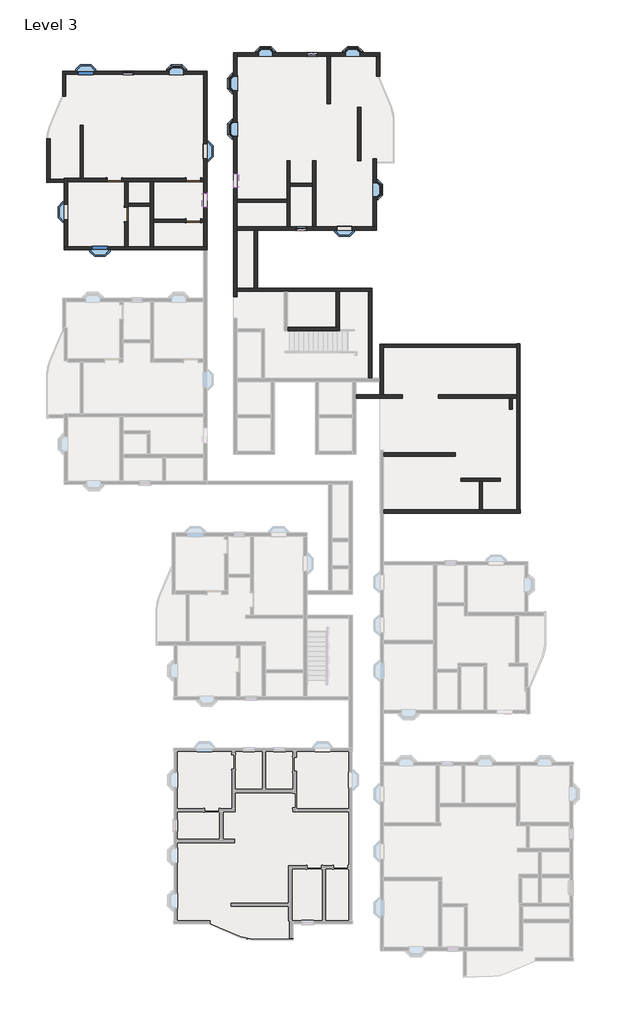
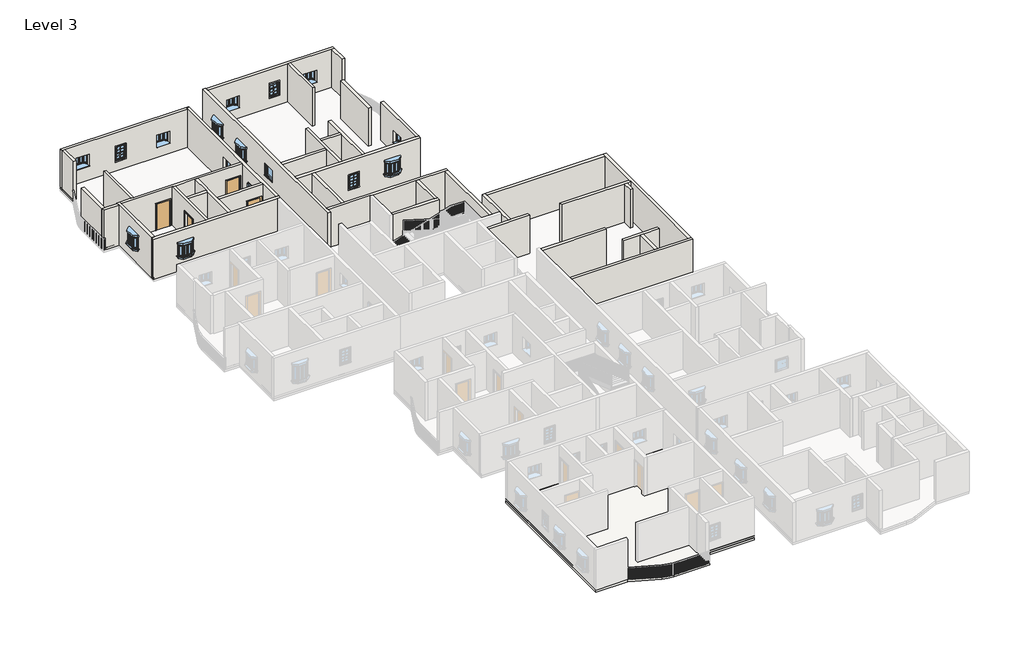
# One storey, part 4 of 14: 39 walls, 16 windows, 4 doors, 1 roof, 1 slab.
# Revit data of these elements (continued)
# Elements 31, 45 (IfcWall, "9\" w") (continued)
#   Top Offset = 0' - 0"
#   Base Offset = 0' - 0"
#   wall height = 10' - 0"
#   Phase Created = New Construction
#   Base Constraint = Level 3
#   Top Constraint = Level 4
#   Materials on its faces: "Default Wall", "Brick, Soldier Course"
# Element 32 (IfcWall, "9\" w")
#   Top Offset = 0' - 0"
#   Base Offset = 0' - 0"
#   wall height = 10' - 0"
#   Phase Created = New Construction
#   Base Constraint = Level 3
#   Top Constraint = Level 4
#   Materials on its faces: "Default Wall", "Grass"
# Element 33 (IfcWall, "9\" w")
#   Top Offset = 0' - 0"
#   Base Offset = 0' - 0"
#   wall height = 10' - 0"
#   Phase Created = New Construction
#   Base Constraint = Level 3
#   Top Constraint = Level 4
#   Materials on its faces: "Default Wall", "Brick, Soldier Course", "Earth"
# Element 34 (IfcWall, "9\" w")
#   Top Offset = 0' - 0"
#   Base Offset = 0' - 0"
#   wall height = 10' - 0"
#   Phase Created = New Construction
#   Base Constraint = Level 3
#   Top Constraint = Level 4
#   Materials on its faces: "Default Wall", "Earth"
# Element 35 (IfcWall, "9\" w")
#   Top Offset = 0' - 0"
#   Base Offset = 0' - 0"
#   wall height = 10' - 0"
#   Phase Created = New Construction
#   Base Constraint = Level 3
#   Top Constraint = Level 4
#   Materials on its faces: "Default Wall", "Parking Stripe"
# Elements 36, 37, 38 (IfcWall, "9\" w")
#   Top Offset = 0' - 0"
#   Base Offset = 0' - 0"
#   wall height = 10' - 0"
#   Phase Created = New Construction
#   Base Constraint = Level 3
#   Top Constraint = Level 4
#   Materials on its faces: "Default Wall", "Window Frame"
# Element 43 (IfcWall, "9\" w")
#   Top Offset = 0' - 0"
#   Base Offset = 0' - 0"
#   wall height = 10' - 0"
#   Phase Created = New Construction
#   Base Constraint = Level 3
#   Top Constraint = Level 4
#   Materials on its faces: "Default Wall", "Parking Stripe", "Default Mass Interior Wall"
# Element 44 (IfcWall, "9\" w")
#   Top Offset = 0' - 0"
#   Base Offset = 0' - 0"
#   wall height = 10' - 0"
#   Phase Created = New Construction
#   Base Constraint = Level 3
#   Top Constraint = Level 4
#   Materials on its faces: "Default Wall", "Parking Stripe", "Brick, Soldier Course"
# Element 46 (IfcWindow, "910x910mm")
#   Mark = "115"
#   Phase Created = New Construction
#   Materials on its faces: "Window Frame", "Glass"
# Element 47 (IfcWindow, "910x910mm")
#   Mark = "116"
#   Phase Created = New Construction
#   Materials on its faces: "Window Frame", "Glass"
# Element 48 (IfcWindow, "910x910mm")
#   Mark = "117"
#   Phase Created = New Construction
#   Materials on its faces: "Window Frame", "Glass"
# Element 49 (IfcWindow, "910x910mm")
#   Mark = "147"
#   Phase Created = New Construction
#   Materials on its faces: "Window Frame", "Glass"
# Element 50 (IfcWindow, "910x910mm")
#   Mark = "148"
#   Phase Created = New Construction
#   Materials on its faces: "Window Frame", "Glass"
# Element 51 (IfcWindow, "910x910mm")
#   Mark = "280"
#   Phase Created = New Construction
#   Materials on its faces: "Window Frame", "Glass"
# Element 52 (IfcWindow, "910x910mm")
#   Mark = "281"
#   Phase Created = New Construction
#   Materials on its faces: "Window Frame", "Glass"
# Element 53 (IfcWindow, "910x910mm")
#   Mark = "292"
#   Phase Created = New Construction
#   Materials on its faces: "Window Frame", "Glass"
# Element 54 (IfcWindow, "910x910mm")
#   Mark = "293"
#   Phase Created = New Construction
#   Materials on its faces: "Window Frame", "Glass"
# Element 55 (IfcWindow, "910x910mm")
#   Mark = "149"
#   Phase Created = New Construction
#   Materials on its faces: "Window Frame", "Glass"
# Element 56 (IfcWindow, "910x910mm")
#   Mark = "150"
#   Phase Created = New Construction
#   Materials on its faces: "Window Frame", "Glass"
# Element 57 (IfcWindow, "Window-Double-Hung : 26\" x 42\"")
#   Mark = "282"
#   Window Inset = 0' - 0"
#   Interior Wall Closure = 0' - 1 1/2"
#   Frame Extension = 0' - 1 1/4"
#   Exterior Wall Closure = 0' - 0 1/2"
#   Interior Trim Visibility = yes
#   Indicator Visibility = yes
#   Exterior Trim Visibility = yes
#   Phase Created = New Construction
#   Materials on its faces: "Wood - Stained", "Glass", "Clad - White"
# Element 58 (IfcWindow, "Window-Double-Hung : 26\" x 42\"")
#   Mark = "294"
#   Window Inset = 0' - 0"
#   Interior Wall Closure = 0' - 1 1/2"
#   Frame Extension = 0' - 1 1/4"
#   Exterior Wall Closure = 0' - 0 1/2"
#   Interior Trim Visibility = yes
#   Indicator Visibility = yes
#   Exterior Trim Visibility = yes
#   Phase Created = New Construction
#   Materials on its faces: "Wood - Stained", "Glass", "Clad - White"
# Element 59 (IfcWindow, "Window-Double-Hung : 26\" x 42\"")
#   Mark = "168"
#   Window Inset = 0' - 0"
#   Interior Wall Closure = 0' - 1 1/2"
#   Frame Extension = 0' - 1 1/4"
#   Exterior Wall Closure = 0' - 0 1/2"
#   Interior Trim Visibility = yes
#   Indicator Visibility = yes
#   Exterior Trim Visibility = yes
#   Phase Created = New Construction
#   Materials on its faces: "Wood - Stained", "Glass", "Clad - White"
# Element 60 (IfcWindow, "Windows_Sgl_w-Glazing_Bars : 910x910mm")
#   Mark = "151"
#   Phase Created = New Construction
#   Materials on its faces: "Window Frame", "Glass"
# Element 61 (IfcWindow, "Windows_Sgl_w-Glazing_Bars : 910x910mm")
#   Mark = "155"
#   Phase Created = New Construction
#   Materials on its faces: "Window Frame", "Glass"
# Materials
#   "Door - Panel": class "Wood", colour RGB 210 159 95, transparency 0, Cost = 0
#   "Door - Frame": colour RGB 118 70 51, transparency 0, Cost = 0
#   "Window Frame": colour RGB 249 249 249, transparency 0
#   "Glass": class "Glass", colour RGB 0 128 192, transparency 0.75, Description = "Soda Lime Glass", Cost = 0
#   "Wood - Stained": class "Wood", colour RGB 224 178 126, transparency 0, Cost = 0
#   "Clad - White": class "Wood", colour RGB 242 242 238, transparency 0, Cost = 0
#   "Default Roof": colour RGB 88 101 114, transparency 0, Cost = 0
#   "Default Floor": colour RGB 128 128 128, transparency 0, Cost = 0
#   "Default Wall": colour RGB 128 128 128, transparency 0, Cost = 0
#   "Grass": class "Generic", colour RGB 104 137 66, transparency 0, Description = "Physical material.", Cost = 0
#   "Parking Stripe": class "Paint", colour RGB 250 250 91, transparency 0, Cost = 0
#   "Carpet (1)": class "Carpet", colour RGB 124 80 67, transparency 0, Description = "Interior finish", Cost = 0
#   "Brick, Soldier Course": class "Masonry", colour RGB 170 98 104, transparency 0, Description = "Common brick soldier coursed", Cost = 0
#   "Default Mass Interior Wall": class "Generic", colour RGB 195 229 126, transparency 0, Cost = 0
#   "Earth": class "Generic", colour RGB 97 75 62, transparency 0, Description = "Soil", Cost = 0
